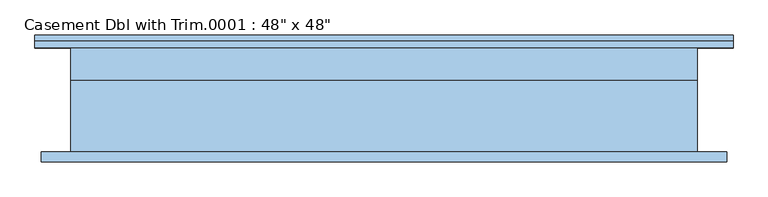
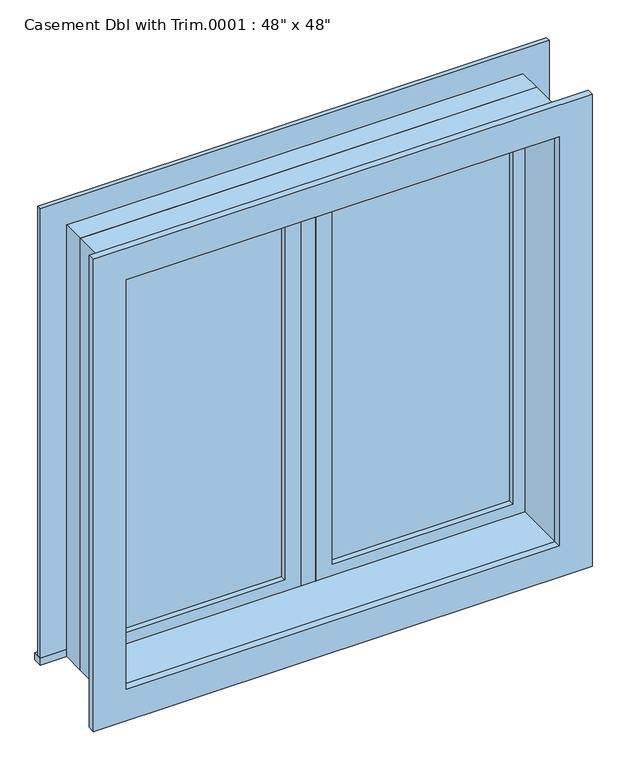
"""IFC4 building model written with IfcOpenShell, lengths in millimetres: window geometry."""

from ifc_helpers import new_model, si_unit, frame, origin, place, context, project, spatial, polyline, outline, extrude, source, transform, mapped, element, save


def window_0862ab64(model_context):
    return source(origin(), model_context, "Body", "SweptSolid", [
        extrude(outline(polyline([(63.5, 85.725), (546.1, 85.725), (546.1, 73.025), (63.5, 73.025), (63.5, 85.725)])), frame((0.0, 0.0, 977.9), z_axis=(0.0, 0.0, 1.0), x_axis=(1.0, 0.0, 0.0)), (0.0, 0.0, 1.0), 1092.2),
        extrude(outline(polyline([(2114.55, 19.05), (933.45, 19.05), (933.45, 590.55), (2114.55, 590.55), (2114.55, 19.05)]), holes=[polyline([(2070.1, 63.5), (2070.1, 546.1), (977.9, 546.1), (977.9, 63.5), (2070.1, 63.5)])]), frame((0.0, 57.15, 0.0), z_axis=(0.0, 1.0, 0.0), x_axis=(0.0, 0.0, 1.0)), (0.0, 0.0, 1.0), 44.45),
        extrude(outline(polyline([(19.05, 57.15), (-19.05, 57.15), (-19.05, 120.65), (19.05, 120.65), (19.05, 57.15)])), frame((0.0, 0.0, 933.45), z_axis=(0.0, 0.0, 1.0), x_axis=(1.0, 0.0, 0.0)), (0.0, 0.0, 1.0), 1181.1),
        extrude(outline(polyline([(-679.45, 146.05), (679.45, 146.05), (679.45, 120.65), (-679.45, 120.65), (-679.45, 146.05)])), frame((0.0, 0.0, 914.4), z_axis=(0.0, 0.0, 1.0), x_axis=(1.0, 0.0, 0.0)), (0.0, 0.0, 1.0), 19.05),
        extrude(outline(polyline([(2114.55, -590.55), (2114.55, 590.55), (933.45, 590.55), (933.45, 679.45), (2203.45, 679.45), (2203.45, -679.45), (933.45, -679.45), (933.45, -590.55), (2114.55, -590.55)])), frame((0.0, 120.65, 0.0), z_axis=(0.0, 1.0, 0.0), x_axis=(0.0, 0.0, 1.0)), (0.0, 0.0, 1.0), 12.7),
        extrude(outline(polyline([(2190.75, 666.75), (2190.75, -666.75), (857.25, -666.75), (857.25, 666.75), (2190.75, 666.75)]), holes=[polyline([(2101.85, 577.85), (946.15, 577.85), (946.15, -577.85), (2101.85, -577.85), (2101.85, 577.85)])]), frame((0.0, -101.6, 0.0), z_axis=(0.0, 1.0, 0.0), x_axis=(0.0, 0.0, 1.0)), (0.0, 0.0, 1.0), 19.05),
        extrude(outline(polyline([(-63.5, 73.025), (-546.1, 73.025), (-546.1, 85.725), (-63.5, 85.725), (-63.5, 73.025)])), frame((0.0, 0.0, 977.9), z_axis=(0.0, 0.0, 1.0), x_axis=(1.0, 0.0, 0.0)), (0.0, 0.0, 1.0), 1092.2),
        extrude(outline(polyline([(2114.55, -590.55), (933.45, -590.55), (933.45, -19.05), (2114.55, -19.05), (2114.55, -590.55)]), holes=[polyline([(2070.1, -546.1), (2070.1, -63.5), (977.9, -63.5), (977.9, -546.1), (2070.1, -546.1)])]), frame((0.0, 57.15, 0.0), z_axis=(0.0, 1.0, 0.0), x_axis=(0.0, 0.0, 1.0)), (0.0, 0.0, 1.0), 44.45),
        extrude(outline(polyline([(2133.6, -609.6), (914.4, -609.6), (914.4, 609.6), (2133.6, 609.6), (2133.6, -609.6)]), holes=[polyline([(2101.85, -577.85), (2101.85, 577.85), (946.15, 577.85), (946.15, -577.85), (2101.85, -577.85)])]), frame((0.0, -82.55, 0.0), z_axis=(0.0, 1.0, 0.0), x_axis=(0.0, 0.0, 1.0)), (0.0, 0.0, 1.0), 139.7),
        extrude(outline(polyline([(2133.6, 609.6), (2133.6, -609.6), (914.4, -609.6), (914.4, 609.6), (2133.6, 609.6)]), holes=[polyline([(2114.55, 590.55), (933.45, 590.55), (933.45, -590.55), (2114.55, -590.55), (2114.55, 590.55)])]), frame((0.0, 57.15, 0.0), z_axis=(0.0, 1.0, 0.0), x_axis=(0.0, 0.0, 1.0)), (0.0, 0.0, 1.0), 63.5),
    ])


if __name__ == "__main__":
    model = new_model("IFC4")
    model_context = context("Model", 3, world=origin())
    ifc_project = project(units=[si_unit("LENGTHUNIT", "METRE", prefix="MILLI")], contexts=[model_context])
    site = spatial("IfcSite", under=ifc_project)
    building = spatial("IfcBuilding", under=site)
    placement = place(None, origin())
    window_shape = window_0862ab64(model_context)
    element("IfcWindow", 1, ObjectType="Casement Dbl with Trim.0001 : 48\" x 48\"", at=placement, inside=building, context=model_context, shape_type="MappedRepresentation", body=[
        mapped(window_shape, transform((0.0, 0.0, 0.0), x_axis=(1.0, 0.0, 0.0), y_axis=(0.0, 1.0, 0.0), z_axis=(0.0, 0.0, 1.0))),
    ])
    save(model, "model.ifc")

# Revit data of these elements
# Type "Casement Dbl with Trim.0001 : 48\" x 48\""
#   Type Mark = "14"
#   Construction Type Id = "GSP4R"
#   Assembly Code = "B2020100"
#   Analytic Construction = "1/8 in Pilkington single glazing"
#   Visual Light Transmittance = 0.9
#   Solar Heat Gain Coefficient = 0.78
#   Heat Transfer Coefficient (U) = 0.6496 BTU/(h·ft²·°F)
#   Height = 4' - 0"
#   Default Sill Height = 3' - 0"
#   Trim Projection - Ext. = 0' - 0 1/2"
#   Trim Projection - Int. = 0' - 0 3/4"
#   Trim Width - Exterior = 0' - 3 1/2"
#   Trim Width - Interior = 0' - 3 1/2"
#   Width = 4' - 0"
#   Window Inset = 0' - 0 3/4"
#   Define Thermal Properties by = 1
#   Glass Pane Material = Glass
#   Sash Material = Sash
#   Trim Exterior Material = Trim
#   Trim Interior Material = Trim
#   Wall Closure = (empty or 0)
# Element 1 (IfcWindow, "Casement Dbl with Trim.0001 : 48\" x 48\"")
#   Materials on its faces: "Sash", "Trim", "Glass"
# Materials
#   "Glass": class "Glass", colour RGB 0 128 192, transparency 0.75, Description = "Soda Lime Glass", Cost = 0
#   "Sash": class "Wood", colour RGB 224 178 126, transparency 0
#   "Trim": class "Wood", colour RGB 224 178 126, transparency 0
